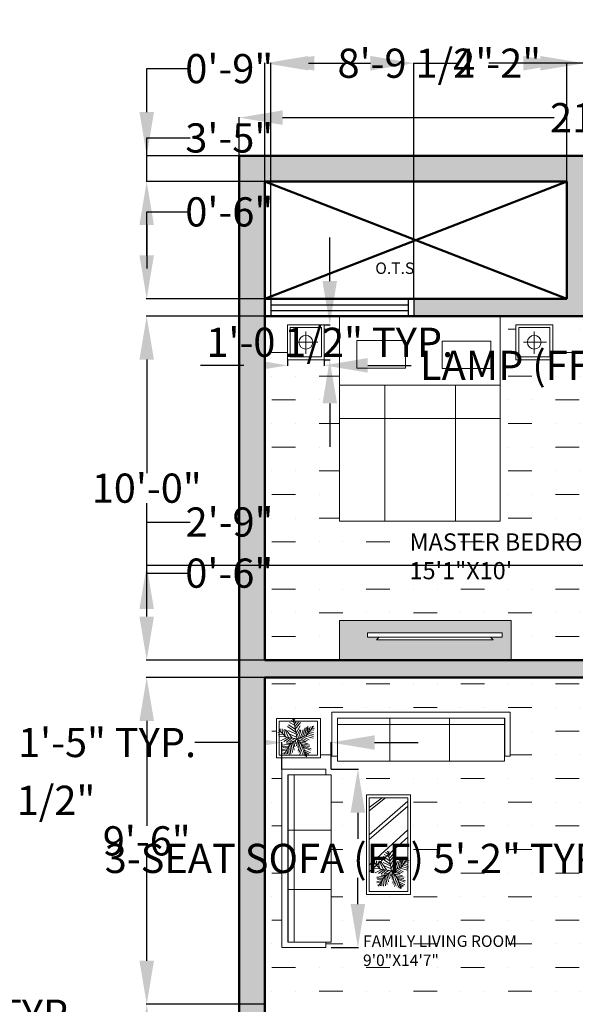
# Model space of a CAD drawing. Units: inches. Extents: x 26 to 14419, y 2 to 3479.
# Tile 8 of 9: x 14003 to 14197, y 3106 to 3449. Entities that reach past the tile are written whole.
import ezdxf

# ---------------------------------------------------------------- set-up
doc = ezdxf.new("R2010")
doc.units = ezdxf.units.IN
doc.header["$MEASUREMENT"] = 0
for name, color, linetype, lineweight in [('A-ANNO-DIMS', 2, 'Continuous', 18), ('A-AREA-IDEN', 7, 'Continuous', 18), ('A-FLOR-PATT', 252, 'Continuous', 13), ('A-FURN', 8, 'Continuous', 18), ('A-GLAZ', 3, 'Continuous', 25), ('A-WALL', 7, 'Continuous', 50), ('L-PLNT', 3, 'Continuous', 13)]:
    doc.layers.add(name, color=color, linetype=linetype, lineweight=lineweight)
doc.styles.get("Standard").update_dxf_attribs({"font": 'arial.ttf'})
doc.dimstyles.get("Standard").update_dxf_attribs({"dimtxt": 10.18, "dimasz": 15.18, "dimexe": 0.18, "dimexo": 0.0625, "dimgap": 0.09, "dimtad": 0, "dimtih": 1, "dimtoh": 1, "dimdec": 0, "dimzin": 0, "dimdsep": 46, "dimlunit": 3, "dimtxsty": 'Standard', "dimcen": 0.09, "dimadec": 0, "dimazin": 0, "dimtfac": 1, "dimtdec": 0, "dimtofl": 0, "dimtmove": 0, "dimatfit": 3, "dimfxl": 1, "dimtolj": 1, "dimtzin": 0, "dimarcsym": 0})

# ---------------------------------------------------------------- blocks, each defined once
blk = doc.blocks.new('*U5')
for p, q in [((-48.585, 21.131), (-49.309, 29.026)), ((-43.513, 28.561), (-42.427, 15.558)), ((-3.665, 19.273), (-27.574, 35.527)), ((-5.114, 28.097), (-24.676, 40.636)), ((-7.288, 39.707), (-21.778, 46.673)), ((-8.737, 47.138), (-17.069, 52.711)), ((-10.186, 53.64), (-13.084, 55.962)), ((0, 0), (-10.5, 57)), ((-9.099, 51.782), (-6.563, 55.962)), ((-7.65, 43.423), (-2.578, 49.46)), ((-5.839, 35.992), (4.667, 48.067)), ((-5.114, 27.632), (10.463, 46.673)), ((-2.941, 16.486), (8.652, 37.85)), ((16.259, 5.805), (23.142, 31.348)), ((22.055, 7.198), (27.489, 32.277)), ((27, 9), (48, 36)), ((27.127, 9.056), (31.112, 35.992)), ((31.836, 30.883), (32.561, 16.486)), ((35.096, 32.741), (37.27, 22.524)), ((38.719, 34.134), (41.979, 28.561)), ((43.791, 29.954), (51.036, 30.883)), ((44.153, 36.456), (45.239, 32.741)), ((-47.498, 19.737), (-55.83, 18.344)), ((-40.615, 13.7), (-55.105, 10.913)), ((-31.5, 4.5), (-52.5, 25.5)), ((-33.37, 6.269), (-52.207, 5.34)), ((-28.299, 3.483), (-47.86, -5.805)), ((-38.442, 26.239), (-34.819, 7.663)), ((-21.416, 3.018), (-38.079, -8.128)), ((-35.544, 28.097), (-24.314, 3.947)), ((0, 0), (-31.5, 4.5)), ((-14.533, 2.09), (-30.834, 25.31)), ((-15.982, 2.09), (-30.11, -9.521)), ((-24.314, 23.917), (-2.941, 13.7)), ((0, 0), (-22.5, -19.5)), ((-6.563, 1.161), (-21.416, -8.128)), ((-20.691, 13.7), (-1.129, 4.876)), ((-1.129, 6.734), (9.014, 26.704)), ((0, 0), (27, 9)), ((0, 0), (18, -22.5)), ((3.942, 1.625), (11.187, 24.381)), ((6.478, 1.625), (26.04, -8.592)), ((10.101, 3.483), (17.708, 26.239)), ((11.187, 3.483), (30.749, -5.805)), ((18.07, 5.805), (35.096, -3.483)), ((24.229, 7.663), (46.688, 1.625)), ((29.662, 12.307), (48.137, 6.269)), ((33.285, 16.486), (48.862, 10.913)), ((36.183, 19.737), (48.137, 17.88)), ((40.53, 25.775), (48.862, 24.846)), ((-17.431, -15.094), (-42.789, -18.809)), ((-24.314, -21.596), (-42.427, -22.06)), ((-26.849, -26.24), (-40.253, -25.775)), ((-22.5, -19.5), (-37.5, -45)), ((-15.257, -12.772), (-30.11, -12.772)), ((-25.038, -23.918), (-22.865, -45.281)), ((-20.691, -18.345), (-17.793, -44.352)), ((-6.563, -5.805), (-19.967, -9.985)), ((-17.069, -15.094), (-12.721, -40.172)), ((-13.446, -11.378), (-8.737, -32.741)), ((-9.461, -8.592), (-6.201, -23.453)), ((-4.752, -3.483), (-3.665, -14.629)), ((2.493, -3.019), (-1.491, -20.202)), ((1.769, -2.555), (24.229, -9.521)), ((5.029, -6.27), (2.131, -25.775)), ((9.014, -11.378), (3.58, -35.992)), ((14.085, -16.951), (6.478, -40.172)), ((7.565, -9.056), (32.198, -14.629)), ((18.07, -22.524), (8.289, -45.745)), ((12.274, -15.094), (36.907, -18.809)), ((16.259, -19.738), (36.183, -22.989)), ((18, -22.5), (27, -52.5)), ((18.433, -22.524), (40.53, -29.026)), ((19.157, -25.311), (38.719, -33.206)), ((-28.299, -29.026), (-42.789, -31.348)), ((-30.834, -34.135), (-42.427, -35.528)), ((-34.457, -39.708), (-40.978, -42.494)), ((-32.646, -36.921), (-31.921, -44.352)), ((-29.023, -30.884), (-27.936, -43.887)), ((20.244, -30.419), (15.897, -44.816)), ((22.78, -37.85), (19.519, -48.532)), ((21.331, -32.741), (39.081, -40.636)), ((22.78, -38.314), (34.372, -44.816)), ((24.591, -45.745), (23.142, -50.854)), ((24.591, -43.423), (30.749, -47.603)), ((26.764, -49.925), (28.213, -50.854))]:
    blk.add_line(p, q)
blk = doc.blocks.new('*D8')
at = {"layer": 'A-ANNO-DIMS', "color": 0, "lineweight": -2, "transparency": 16777216}
for p, q in [((14079.64, 3401.78), (14079.64, 3415.17)), ((14094.82, 3414.99), (14189.53, 3414.99)), ((14327.46, 3414.99), (14232.76, 3414.99)), ((14342.64, 3401.78), (14342.64, 3415.17))]:
    blk.add_line(p, q, dxfattribs=at)
at = {"layer": 'A-ANNO-DIMS', "color": 0, "transparency": 16777216}
for points in [[(14094.82, 3417.52), (14094.82, 3412.46), (14079.64, 3414.99)], [(14327.46, 3417.52), (14327.46, 3412.46), (14342.64, 3414.99)]]:
    blk.add_solid(points, dxfattribs=at)
at = {"layer": 'Defpoints', "color": 0, "transparency": 16777216}
for p in [(14342.64, 3414.99), (14079.64, 3401.72), (14342.64, 3401.72)]:
    blk.add_point(p, dxfattribs=at)
at = {"layer": 'A-ANNO-DIMS', "color": 0, "transparency": 16777216, "insert": (14211.14, 3414.99), "char_height": 10.18, "attachment_point": 5}
blk.add_mtext('\\A1;21\'-11"', dxfattribs=at)
blk = doc.blocks.new('SOFA-3SEAT-FF')
for points in [[(1.92, 15.07), (1.92, 1.81), (0, 1.81), (0, 17.18), (1.92, 17.18)], [(1.92, 17.18), (62.18, 17.18)], [(60.26, 17.18), (62.18, 17.18), (62.18, 1.81), (60.26, 1.81), (60.26, 15.07)], [(60.26, 15.07), (1.92, 15.07)]]:
    blk.add_lwpolyline(points)
blk.add_lwpolyline([(1.92, 15.02), (60.19, 15.02), (60.19, 0), (1.92, 0)], close=True)
blk = doc.blocks.new('LAMP-FF')
for p, q in [((6.41, 9.87), (6.41, 2.06)), ((2.67, 6.13), (10.62, 6.13))]:
    blk.add_line(p, q)
for points in [[(0, 12.26), (12.83, 12.26), (12.83, 0), (0, 0)], [(1, 11.26), (11.83, 11.26), (11.83, 1), (1, 1)]]:
    blk.add_lwpolyline(points, close=True)
blk.add_circle((6.41, 6.13), 2.41)
blk = doc.blocks.new('*D33')
at = {"layer": 'A-ANNO-DIMS', "color": 0, "lineweight": -2, "transparency": 16777216}
for p, q in [((14111.8, 3187.7), (14121.24, 3187.7)), ((14121.06, 3172.52), (14121.06, 3163.38)), ((14121.06, 3140.7), (14121.06, 3149.84)), ((14111.8, 3125.52), (14121.24, 3125.52))]:
    blk.add_line(p, q, dxfattribs=at)
at = {"layer": 'A-ANNO-DIMS', "color": 0, "transparency": 16777216}
for points in [[(14118.53, 3172.52), (14123.59, 3172.52), (14121.06, 3187.7)], [(14118.53, 3140.7), (14123.59, 3140.7), (14121.06, 3125.52)]]:
    blk.add_solid(points, dxfattribs=at)
at = {"layer": 'Defpoints', "color": 0, "transparency": 16777216}
for p in [(14111.74, 3187.7), (14121.06, 3187.7), (14111.74, 3125.52)]:
    blk.add_point(p, dxfattribs=at)
at = {"layer": 'A-ANNO-DIMS', "color": 0, "transparency": 16777216, "insert": (14121.06, 3156.61), "char_height": 10.18, "attachment_point": 5}
blk.add_mtext('\\A1;3-SEAT SOFA (FF) 5\'-2" TYP.', dxfattribs=at)
blk = doc.blocks.new('*D34')
at = {"layer": 'A-ANNO-DIMS', "color": 0, "lineweight": -2, "transparency": 16777216}
for p, q in [((14079.38, 3197.03), (14064.2, 3197.03)), ((14094.56, 3187.76), (14094.56, 3197.21)), ((14111.74, 3187.76), (14111.74, 3197.21)), ((14126.92, 3197.03), (14142.1, 3197.03))]:
    blk.add_line(p, q, dxfattribs=at)
at = {"layer": 'A-ANNO-DIMS', "color": 0, "transparency": 16777216}
for points in [[(14079.38, 3199.56), (14079.38, 3194.5), (14094.56, 3197.03)], [(14126.92, 3199.56), (14126.92, 3194.5), (14111.74, 3197.03)]]:
    blk.add_solid(points, dxfattribs=at)
at = {"layer": 'Defpoints', "color": 0, "transparency": 16777216}
for p in [(14094.56, 3197.03), (14094.56, 3187.7), (14111.74, 3187.7)]:
    blk.add_point(p, dxfattribs=at)
at = {"layer": 'A-ANNO-DIMS', "color": 0, "transparency": 16777216, "insert": (14033.56, 3197.03), "char_height": 10.18, "attachment_point": 5}
blk.add_mtext('\\A1;1\'-5" TYP.', dxfattribs=at)
blk = doc.blocks.new('*D37')
at = {"layer": 'A-ANNO-DIMS', "color": 0, "lineweight": -2, "transparency": 16777216}
for p, q in [((14081.32, 3328.58), (14066.14, 3328.58)), ((14096.5, 3330.45), (14096.5, 3328.4)), ((14109.33, 3330.45), (14109.33, 3328.4)), ((14124.51, 3328.58), (14139.69, 3328.58))]:
    blk.add_line(p, q, dxfattribs=at)
at = {"layer": 'A-ANNO-DIMS', "color": 0, "transparency": 16777216}
for points in [[(14081.32, 3331.11), (14081.32, 3326.05), (14096.5, 3328.58)], [(14124.51, 3331.11), (14124.51, 3326.05), (14109.33, 3328.58)]]:
    blk.add_solid(points, dxfattribs=at)
at = {"layer": 'Defpoints', "color": 0, "transparency": 16777216}
for p in [(14096.5, 3330.51), (14109.33, 3330.51), (14109.33, 3328.58)]:
    blk.add_point(p, dxfattribs=at)
at = {"layer": 'A-ANNO-DIMS', "color": 0, "transparency": 16777216, "insert": (14207.31, 3328.58), "char_height": 10.18, "attachment_point": 5}
blk.add_mtext('\\A1;LAMP (FF) 1\'-1" TYP.', dxfattribs=at)
blk = doc.blocks.new('*D38')
at = {"layer": 'A-ANNO-DIMS', "color": 0, "lineweight": -2, "transparency": 16777216}
for p, q in [((14111.25, 3357.95), (14111.25, 3373.13)), ((14109.39, 3342.77), (14111.43, 3342.77)), ((14109.39, 3330.51), (14111.43, 3330.51)), ((14111.25, 3315.33), (14111.25, 3300.15))]:
    blk.add_line(p, q, dxfattribs=at)
at = {"layer": 'A-ANNO-DIMS', "color": 0, "transparency": 16777216}
for points in [[(14108.72, 3357.95), (14113.78, 3357.95), (14111.25, 3342.77)], [(14108.72, 3315.33), (14113.78, 3315.33), (14111.25, 3330.51)]]:
    blk.add_solid(points, dxfattribs=at)
at = {"layer": 'Defpoints', "color": 0, "transparency": 16777216}
for p in [(14109.33, 3342.77), (14111.25, 3342.77), (14109.33, 3330.51)]:
    blk.add_point(p, dxfattribs=at)
at = {"layer": 'A-ANNO-DIMS', "color": 0, "transparency": 16777216, "insert": (14111.25, 3336.64), "char_height": 10.18, "attachment_point": 5}
blk.add_mtext('\\A1;1\'-0 1/2" TYP.', dxfattribs=at)
blk = doc.blocks.new('*D46')
at = {"layer": 'A-ANNO-DIMS', "color": 0, "lineweight": -2, "transparency": 16777216}
for p, q in [((13878.23, 3102.3), (13863.05, 3102.3)), ((13893.41, 3104.57), (13893.41, 3102.12)), ((13907.93, 3104.57), (13907.93, 3102.12)), ((13923.11, 3102.3), (13938.29, 3102.3))]:
    blk.add_line(p, q, dxfattribs=at)
at = {"layer": 'A-ANNO-DIMS', "color": 0, "transparency": 16777216}
for points in [[(13878.23, 3104.83), (13878.23, 3099.77), (13893.41, 3102.3)], [(13923.11, 3104.83), (13923.11, 3099.77), (13907.93, 3102.3)]]:
    blk.add_solid(points, dxfattribs=at)
at = {"layer": 'Defpoints', "color": 0, "transparency": 16777216}
for p in [(13893.41, 3104.63), (13907.93, 3104.63), (13907.93, 3102.3)]:
    blk.add_point(p, dxfattribs=at)
at = {"layer": 'A-ANNO-DIMS', "color": 0, "transparency": 16777216, "insert": (13980.79, 3102.3), "char_height": 10.18, "attachment_point": 5}
blk.add_mtext('\\A1;1\'-2 1/2" TYP.', dxfattribs=at)
blk = doc.blocks.new('*D83')
at = {"layer": 'A-ANNO-DIMS', "color": 0, "lineweight": -2, "transparency": 16777216}
for p, q in [((13953.59, 3161.69), (13953.59, 3176.87)), ((13953.59, 3176.87), (13968.77, 3176.87)), ((13883.2, 3161.69), (13953.77, 3161.69)), ((13953.59, 3142.18), (13953.59, 3146.51)), ((13883.2, 3127), (13953.77, 3127))]:
    blk.add_line(p, q, dxfattribs=at)
at = {"layer": 'A-ANNO-DIMS', "color": 0, "transparency": 16777216}
for points in [[(13951.06, 3146.51), (13956.12, 3146.51), (13953.59, 3161.69)], [(13951.06, 3142.18), (13956.12, 3142.18), (13953.59, 3127)]]:
    blk.add_solid(points, dxfattribs=at)
at = {"layer": 'Defpoints', "color": 0, "transparency": 16777216}
for p in [(13883.14, 3161.69), (13953.59, 3161.69), (13883.14, 3127)]:
    blk.add_point(p, dxfattribs=at)
at = {"layer": 'A-ANNO-DIMS', "color": 0, "transparency": 16777216, "insert": (13998.29, 3176.87), "char_height": 10.18, "attachment_point": 5}
blk.add_mtext('\\A1;2\'-10 1/2"', dxfattribs=at)
blk = doc.blocks.new('*D92')
at = {"layer": 'A-ANNO-DIMS', "color": 0, "lineweight": -2, "transparency": 16777216}
for p, q in [((14088.58, 3105.72), (14047.21, 3105.72)), ((14047.39, 3090.54), (14047.39, 3081.01)), ((14047.39, 3060.9), (14047.39, 3070.43)), ((14088.58, 3045.72), (14047.21, 3045.72))]:
    blk.add_line(p, q, dxfattribs=at)
at = {"layer": 'A-ANNO-DIMS', "color": 0, "transparency": 16777216}
for points in [[(14044.86, 3090.54), (14049.92, 3090.54), (14047.39, 3105.72)], [(14044.86, 3060.9), (14049.92, 3060.9), (14047.39, 3045.72)]]:
    blk.add_solid(points, dxfattribs=at)
at = {"layer": 'Defpoints', "color": 0, "transparency": 16777216}
for p in [(14047.39, 3105.72), (14088.64, 3105.72), (14088.64, 3045.72)]:
    blk.add_point(p, dxfattribs=at)
at = {"layer": 'A-ANNO-DIMS', "color": 0, "transparency": 16777216, "insert": (14047.39, 3075.72), "char_height": 10.18, "attachment_point": 5}
blk.add_mtext('\\A1;5\'-0"', dxfattribs=at)
blk = doc.blocks.new('*D93')
at = {"layer": 'A-ANNO-DIMS', "color": 0, "lineweight": -2, "transparency": 16777216}
for p, q in [((14088.58, 3219.75), (14047.21, 3219.75)), ((14047.39, 3204.57), (14047.39, 3168.02)), ((14047.39, 3120.9), (14047.39, 3157.44)), ((14088.58, 3105.72), (14047.21, 3105.72))]:
    blk.add_line(p, q, dxfattribs=at)
at = {"layer": 'A-ANNO-DIMS', "color": 0, "transparency": 16777216}
for points in [[(14044.86, 3204.57), (14049.92, 3204.57), (14047.39, 3219.75)], [(14044.86, 3120.9), (14049.92, 3120.9), (14047.39, 3105.72)]]:
    blk.add_solid(points, dxfattribs=at)
at = {"layer": 'Defpoints', "color": 0, "transparency": 16777216}
for p in [(14047.39, 3219.75), (14088.64, 3219.75), (14088.64, 3105.72)]:
    blk.add_point(p, dxfattribs=at)
at = {"layer": 'A-ANNO-DIMS', "color": 0, "transparency": 16777216, "insert": (14047.39, 3162.73), "char_height": 10.18, "attachment_point": 5}
blk.add_mtext('\\A1;9\'-6"', dxfattribs=at)
blk = doc.blocks.new('*D94')
at = {"layer": 'A-ANNO-DIMS', "color": 0, "lineweight": -2, "transparency": 16777216}
for p, q in [((14047.39, 3240.93), (14047.39, 3256.11)), ((14047.39, 3256.11), (14062.57, 3256.11)), ((14088.58, 3225.75), (14047.21, 3225.75)), ((14088.58, 3219.75), (14047.21, 3219.75)), ((14047.39, 3204.57), (14047.39, 3189.39))]:
    blk.add_line(p, q, dxfattribs=at)
at = {"layer": 'A-ANNO-DIMS', "color": 0, "transparency": 16777216}
for points in [[(14044.86, 3240.93), (14049.92, 3240.93), (14047.39, 3225.75)], [(14044.86, 3204.57), (14049.92, 3204.57), (14047.39, 3219.75)]]:
    blk.add_solid(points, dxfattribs=at)
at = {"layer": 'Defpoints', "color": 0, "transparency": 16777216}
for p in [(14047.39, 3225.75), (14088.64, 3225.75), (14088.64, 3219.75)]:
    blk.add_point(p, dxfattribs=at)
at = {"layer": 'A-ANNO-DIMS', "color": 0, "transparency": 16777216, "insert": (14076.19, 3256.11), "char_height": 10.18, "attachment_point": 5}
blk.add_mtext('\\A1;0\'-6"', dxfattribs=at)
blk = doc.blocks.new('*D95')
at = {"layer": 'A-ANNO-DIMS', "color": 0, "lineweight": -2, "transparency": 16777216}
for p, q in [((14088.58, 3345.75), (14047.21, 3345.75)), ((14047.39, 3330.57), (14047.39, 3291.03)), ((14047.39, 3240.93), (14047.39, 3280.46)), ((14088.58, 3225.75), (14047.21, 3225.75))]:
    blk.add_line(p, q, dxfattribs=at)
at = {"layer": 'A-ANNO-DIMS', "color": 0, "transparency": 16777216}
for points in [[(14044.86, 3330.57), (14049.92, 3330.57), (14047.39, 3345.75)], [(14044.86, 3240.93), (14049.92, 3240.93), (14047.39, 3225.75)]]:
    blk.add_solid(points, dxfattribs=at)
at = {"layer": 'Defpoints', "color": 0, "transparency": 16777216}
for p in [(14047.39, 3345.75), (14088.64, 3345.75), (14088.64, 3225.75)]:
    blk.add_point(p, dxfattribs=at)
at = {"layer": 'A-ANNO-DIMS', "color": 0, "transparency": 16777216, "insert": (14047.39, 3285.75), "char_height": 10.18, "attachment_point": 5}
blk.add_mtext('\\A1;10\'-0"', dxfattribs=at)
blk = doc.blocks.new('*D96')
at = {"layer": 'A-ANNO-DIMS', "color": 0, "lineweight": -2, "transparency": 16777216}
for p, q in [((14047.39, 3366.93), (14047.39, 3382.11)), ((14047.39, 3382.11), (14062.57, 3382.11)), ((14088.58, 3351.75), (14047.21, 3351.75)), ((14088.58, 3345.75), (14047.21, 3345.75)), ((14047.39, 3330.57), (14047.39, 3315.39))]:
    blk.add_line(p, q, dxfattribs=at)
at = {"layer": 'A-ANNO-DIMS', "color": 0, "transparency": 16777216}
for points in [[(14044.86, 3366.93), (14049.92, 3366.93), (14047.39, 3351.75)], [(14044.86, 3330.57), (14049.92, 3330.57), (14047.39, 3345.75)]]:
    blk.add_solid(points, dxfattribs=at)
at = {"layer": 'Defpoints', "color": 0, "transparency": 16777216}
for p in [(14047.39, 3351.75), (14088.64, 3351.75), (14088.64, 3345.75)]:
    blk.add_point(p, dxfattribs=at)
at = {"layer": 'A-ANNO-DIMS', "color": 0, "transparency": 16777216, "insert": (14076.19, 3382.11), "char_height": 10.18, "attachment_point": 5}
blk.add_mtext('\\A1;0\'-6"', dxfattribs=at)
blk = doc.blocks.new('*D97')
at = {"layer": 'A-ANNO-DIMS', "color": 0, "lineweight": -2, "transparency": 16777216}
for p, q in [((14047.39, 3392.72), (14047.39, 3407.9)), ((14047.39, 3407.9), (14062.57, 3407.9)), ((14088.58, 3392.72), (14047.21, 3392.72)), ((14047.39, 3366.93), (14047.39, 3377.54)), ((14088.58, 3351.75), (14047.21, 3351.75))]:
    blk.add_line(p, q, dxfattribs=at)
at = {"layer": 'A-ANNO-DIMS', "color": 0, "transparency": 16777216}
for points in [[(14044.86, 3377.54), (14049.92, 3377.54), (14047.39, 3392.72)], [(14044.86, 3366.93), (14049.92, 3366.93), (14047.39, 3351.75)]]:
    blk.add_solid(points, dxfattribs=at)
at = {"layer": 'Defpoints', "color": 0, "transparency": 16777216}
for p in [(14047.39, 3392.72), (14088.64, 3392.72), (14088.64, 3351.75)]:
    blk.add_point(p, dxfattribs=at)
at = {"layer": 'A-ANNO-DIMS', "color": 0, "transparency": 16777216, "insert": (14076.19, 3407.9), "char_height": 10.18, "attachment_point": 5}
blk.add_mtext('\\A1;3\'-5"', dxfattribs=at)
blk = doc.blocks.new('*D98')
at = {"layer": 'A-ANNO-DIMS', "color": 0, "lineweight": -2, "transparency": 16777216}
for p, q in [((14047.39, 3416.9), (14047.39, 3432.08)), ((14047.39, 3432.08), (14062.57, 3432.08)), ((14079.58, 3401.72), (14047.21, 3401.72)), ((14088.58, 3392.72), (14047.21, 3392.72)), ((14047.39, 3377.54), (14047.39, 3362.36))]:
    blk.add_line(p, q, dxfattribs=at)
at = {"layer": 'A-ANNO-DIMS', "color": 0, "transparency": 16777216}
for points in [[(14044.86, 3416.9), (14049.92, 3416.9), (14047.39, 3401.72)], [(14044.86, 3377.54), (14049.92, 3377.54), (14047.39, 3392.72)]]:
    blk.add_solid(points, dxfattribs=at)
at = {"layer": 'Defpoints', "color": 0, "transparency": 16777216}
for p in [(14047.39, 3401.72), (14079.64, 3401.72), (14088.64, 3392.72)]:
    blk.add_point(p, dxfattribs=at)
at = {"layer": 'A-ANNO-DIMS', "color": 0, "transparency": 16777216, "insert": (14076.19, 3432.08), "char_height": 10.18, "attachment_point": 5}
blk.add_mtext('\\A1;0\'-9"', dxfattribs=at)
blk = doc.blocks.new('*D106')
at = {"layer": 'A-ANNO-DIMS', "color": 0, "lineweight": -2, "transparency": 16777216}
for p, q in [((14088.64, 3392.78), (14088.64, 3434.15)), ((14103.82, 3433.97), (14115.8, 3433.97)), ((14178.75, 3433.97), (14166.77, 3433.97)), ((14193.93, 3392.78), (14193.93, 3434.15))]:
    blk.add_line(p, q, dxfattribs=at)
at = {"layer": 'A-ANNO-DIMS', "color": 0, "transparency": 16777216}
for points in [[(14103.82, 3436.5), (14103.82, 3431.44), (14088.64, 3433.97)], [(14178.75, 3436.5), (14178.75, 3431.44), (14193.93, 3433.97)]]:
    blk.add_solid(points, dxfattribs=at)
at = {"layer": 'Defpoints', "color": 0, "transparency": 16777216}
for p in [(14193.93, 3433.97), (14088.64, 3392.72), (14193.93, 3392.72)]:
    blk.add_point(p, dxfattribs=at)
at = {"layer": 'A-ANNO-DIMS', "color": 0, "transparency": 16777216, "insert": (14141.28, 3433.97), "char_height": 10.18, "attachment_point": 5}
blk.add_mtext('\\A1;8\'-9 1/2"', dxfattribs=at)
blk = doc.blocks.new('*D107')
at = {"layer": 'A-ANNO-DIMS', "color": 0, "lineweight": -2, "transparency": 16777216}
for p, q in [((14184.75, 3433.97), (14169.57, 3433.97)), ((14199.93, 3392.78), (14199.93, 3434.15)), ((14257.64, 3392.78), (14257.64, 3434.15)), ((14272.82, 3433.97), (14288, 3433.97))]:
    blk.add_line(p, q, dxfattribs=at)
at = {"layer": 'A-ANNO-DIMS', "color": 0, "transparency": 16777216}
for points in [[(14184.75, 3436.5), (14184.75, 3431.44), (14199.93, 3433.97)], [(14272.82, 3436.5), (14272.82, 3431.44), (14257.64, 3433.97)]]:
    blk.add_solid(points, dxfattribs=at)
at = {"layer": 'Defpoints', "color": 0, "transparency": 16777216}
for p in [(14257.64, 3433.97), (14199.93, 3392.72), (14257.64, 3392.72)]:
    blk.add_point(p, dxfattribs=at)
at = {"layer": 'A-ANNO-DIMS', "color": 0, "transparency": 16777216, "insert": (14228.78, 3433.97), "char_height": 10.18, "attachment_point": 5}
blk.add_mtext('\\A1;4\'-9 1/2"', dxfattribs=at)
blk = doc.blocks.new('*D109')
at = {"layer": 'A-ANNO-DIMS', "color": 0, "lineweight": -2, "transparency": 16777216}
for p, q in [((14199.604862, 3433.969118), (14184.424862, 3433.969118)), ((14214.784862, 3401.781618), (14214.784862, 3434.149118)), ((14242.784862, 3401.781618), (14242.784862, 3434.149118)), ((14257.964862, 3433.969118), (14273.144862, 3433.969118))]:
    blk.add_line(p, q, dxfattribs=at)
at = {"layer": 'A-ANNO-DIMS', "color": 0, "transparency": 16777216}
for points in [[(14199.604862, 3436.499118), (14199.604862, 3431.439118), (14214.784862, 3433.969118)], [(14257.964862, 3436.499118), (14257.964862, 3431.439118), (14242.784862, 3433.969118)]]:
    blk.add_solid(points, dxfattribs=at)
at = {"layer": 'Defpoints', "color": 0, "transparency": 16777216}
for p in [(14242.784862, 3433.969118), (14214.784862, 3401.719118), (14242.784862, 3401.719118)]:
    blk.add_point(p, dxfattribs=at)
at = {"layer": 'A-ANNO-DIMS', "color": 0, "transparency": 16777216, "insert": (14228.784862, 3433.969118), "char_height": 10.18, "attachment_point": 5}
blk.add_mtext('\\A1;2\'-4"', dxfattribs=at)
blk = doc.blocks.new('*D115')
at = {"layer": 'A-ANNO-DIMS', "color": 0, "lineweight": -2, "transparency": 16777216}
for p, q in [((14090.64, 3351.81), (14090.64, 3434.15)), ((14105.82, 3433.97), (14125.46, 3433.97)), ((14140.64, 3351.81), (14140.64, 3434.15)), ((14140.64, 3433.97), (14155.82, 3433.97))]:
    blk.add_line(p, q, dxfattribs=at)
at = {"layer": 'A-ANNO-DIMS', "color": 0, "transparency": 16777216}
for points in [[(14105.82, 3436.5), (14105.82, 3431.44), (14090.64, 3433.97)], [(14125.46, 3436.5), (14125.46, 3431.44), (14140.64, 3433.97)]]:
    blk.add_solid(points, dxfattribs=at)
at = {"layer": 'Defpoints', "color": 0, "transparency": 16777216}
for p in [(14140.64, 3433.97), (14090.64, 3351.75), (14140.64, 3351.75)]:
    blk.add_point(p, dxfattribs=at)
at = {"layer": 'A-ANNO-DIMS', "color": 0, "transparency": 16777216, "insert": (14169.65, 3433.97), "char_height": 10.18, "attachment_point": 5}
blk.add_mtext('\\A1;4\'-2"', dxfattribs=at)
blk = doc.blocks.new('*D118')
at = {"layer": 'A-ANNO-DIMS', "color": 0, "lineweight": -2, "transparency": 16777216}
for p, q in [((14202.46, 3433.97), (14187.28, 3433.97)), ((14217.64, 3164.78), (14217.64, 3434.15)), ((14227.64, 3164.78), (14227.64, 3434.15)), ((14242.82, 3433.97), (14258, 3433.97))]:
    blk.add_line(p, q, dxfattribs=at)
at = {"layer": 'A-ANNO-DIMS', "color": 0, "transparency": 16777216}
for points in [[(14202.46, 3436.5), (14202.46, 3431.44), (14217.64, 3433.97)], [(14242.82, 3436.5), (14242.82, 3431.44), (14227.64, 3433.97)]]:
    blk.add_solid(points, dxfattribs=at)
at = {"layer": 'Defpoints', "color": 0, "transparency": 16777216}
for p in [(14227.64, 3433.97), (14217.64, 3164.72), (14227.64, 3164.72)]:
    blk.add_point(p, dxfattribs=at)
at = {"layer": 'A-ANNO-DIMS', "color": 0, "transparency": 16777216, "insert": (14275.58, 3433.97), "char_height": 10.18, "attachment_point": 5}
blk.add_mtext('\\A1;0\'-10"', dxfattribs=at)
blk = doc.blocks.new('*D120')
at = {"layer": 'A-ANNO-DIMS', "color": 0, "lineweight": -2, "transparency": 16777216}
for p, q in [((14047.39, 3258.75), (14047.39, 3273.93)), ((14047.39, 3273.93), (14062.57, 3273.93)), ((14254.58, 3258.75), (14047.21, 3258.75)), ((14047.39, 3240.93), (14047.39, 3243.57)), ((14257.58, 3225.75), (14047.21, 3225.75))]:
    blk.add_line(p, q, dxfattribs=at)
at = {"layer": 'A-ANNO-DIMS', "color": 0, "transparency": 16777216}
for points in [[(14044.86, 3243.57), (14049.92, 3243.57), (14047.39, 3258.75)], [(14044.86, 3240.93), (14049.92, 3240.93), (14047.39, 3225.75)]]:
    blk.add_solid(points, dxfattribs=at)
at = {"layer": 'Defpoints', "color": 0, "transparency": 16777216}
for p in [(14047.39, 3258.75), (14254.64, 3258.75), (14257.64, 3225.75)]:
    blk.add_point(p, dxfattribs=at)
at = {"layer": 'A-ANNO-DIMS', "color": 0, "transparency": 16777216, "insert": (14076.28, 3273.93), "char_height": 10.18, "attachment_point": 5}
blk.add_mtext('\\A1;2\'-9"', dxfattribs=at)

msp = doc.modelspace()

# ---------------------------------------------------------------- hatches: boundary and pattern name
at = {"layer": 'A-FLOR-PATT'}
h = msp.add_hatch(color=256, dxfattribs=at)
h.dxf.hatch_style = 1
h.paths.add_polyline_path([(13922.09, 3432), (13659.09, 3432), (13659.09, 2842), (13668.09, 2842), (13668.09, 2851), (13668.09, 2899), (13668.09, 2908), (13668.09, 3076), (13706.09, 3076), (13706.09, 3085), (13668.09, 3085), (13668.09, 3249), (13712.76, 3249), (13712.76, 3255), (13668.09, 3255), (13668.09, 3375), (13720.94, 3375), (13720.94, 3378, -0.017236), (13720.94, 3380), (13720.94, 3381), (13668.09, 3381), (13668.09, 3423), (13784.09, 3423), (13784.09, 3381), (13753.94, 3381), (13753.94, 3375), (13784.09, 3375), (13784.09, 3255), (13758.77, 3255), (13758.77, 3249), (13784.09, 3249), (13793.09, 3249), (13793.09, 3255), (13793.09, 3423), (13913.09, 3423), (13913.09, 3255), (13832.09, 3255), (13832.09, 3254, -0.014283), (13832.09, 3252), (13832.09, 3249), (13836.57, 3249), (13836.57, 3234), (13839.57, 3234, -0.017236), (13841.57, 3234), (13842.57, 3234), (13842.57, 3249), (13913.09, 3249), (13913.09, 3201), (13892.46, 3201), (13793.09, 3201), (13784.09, 3201), (13784.09, 3195), (13793.09, 3195), (13913.09, 3195), (13913.09, 3127), (13922.09, 3127)])
h.paths.add_polyline_path([(13922.09, 3013.5), (13913.09, 3013.5), (13913.09, 2908), (13892.09, 2908), (13892.09, 2899), (13913.09, 2899), (13913.09, 2851), (13793.09, 2851), (13784.09, 2851), (13784.09, 2842), (13922.09, 2842)], flags=17)
h.paths.add_polyline_path([(13793.09, 3085), (13784.09, 3085), (13784.09, 3076), (13784.09, 3071.08), (13784.09, 3066.17), (13784.09, 2908), (13784.09, 2899.07), (13793.09, 2899), (13802.09, 2899), (13814.09, 2899), (13814.09, 2908), (13793.09, 2908)], flags=17)
h.paths.add_polyline_path([(14342.64, 3401.72), (14242.78, 3401.72), (14242.78, 3392.72), (14257.64, 3392.72), (14257.64, 3351.75), (14257.64, 3345.75), (14257.64, 3330.73), (14263.64, 3330.73), (14263.64, 3392.72), (14333.64, 3392.72), (14333.64, 3284.72), (14302.92, 3284.72), (14302.92, 3281.72, -0.022645), (14302.92, 3279.12), (14302.92, 3278.72), (14333.64, 3278.72), (14333.64, 3170.72), (14316.1, 3170.72), (14263.64, 3170.72), (14263.64, 3278.72), (14269.92, 3278.72), (14269.92, 3284.72), (14263.64, 3284.72), (14257.64, 3284.72), (14257.64, 3225.75), (14257.64, 3219.75), (14257.64, 3164.72), (14333.64, 3164.72), (14333.64, 3110.37), (14210.01, 3110.37), (14210.01, 3104.37), (14257.64, 3104.37), (14257.64, 3024), (14263.64, 3024), (14263.64, 3039.72), (14263.64, 3104.37), (14333.64, 3104.37), (14333.64, 3045.72), (14333.64, 3039.72), (14333.64, 2967.72), (14296.64, 2967.72), (14296.64, 2964.72, -0.017236), (14296.64, 2962.72), (14296.64, 2961.72), (14333.64, 2961.72), (14333.64, 2882.72), (14312.64, 2882.72), (14312.64, 2873.72), (14333.64, 2873.72), (14333.64, 2820.72), (14333.64, 2811.72), (14342.64, 2811.72)])
h.paths.add_polyline_path([(14088.64, 3219.75), (14218.64, 3219.75), (14218.64, 3222.75, -0.014283), (14218.64, 3224.75), (14218.64, 3225.75), (14088.64, 3225.75), (14088.64, 3345.75), (14088.64, 3351.75), (14088.64, 3392.72), (14193.93, 3392.72), (14193.93, 3351.75), (14140.64, 3351.75), (14140.64, 3345.75), (14170.7, 3345.75), (14218.64, 3345.75), (14218.64, 3348.75, -0.014283), (14218.64, 3350.75), (14218.64, 3351.75), (14199.93, 3351.75), (14199.93, 3392.72), (14214.78, 3392.72), (14214.78, 3401.72), (14079.64, 3401.72), (14079.64, 2811.72), (14088.64, 2811.72), (14088.64, 2820.72), (14088.64, 2873.72), (14116.21, 2873.72), (14116.21, 2876.57), (14116.21, 2882.72), (14088.64, 2882.72), (14088.64, 3039.72), (14216.01, 3039.72), (14216.01, 3065.37), (14215.01, 3065.37, -0.014283), (14213.01, 3065.37), (14210.01, 3065.37), (14210.01, 3045.72), (14154.64, 3045.72), (14148.64, 3045.72), (14088.64, 3045.72)])
h.paths.add_polyline_path([(14284.64, 2882.72), (14263.64, 2882.72), (14263.64, 2961.72), (14263.64, 2967.72), (14257.64, 2967.72), (14257.64, 2956.69), (14257.64, 2916.18), (14257.64, 2882.72), (14249.61, 2882.72), (14249.61, 2873.72), (14284.64, 2873.72)], flags=17)
h.paths.add_polyline_path([(14202.78, 2882.72), (14189.55, 2882.72), (14189.55, 2879.95), (14189.55, 2873.72), (14202.78, 2873.72)], flags=17)
h = msp.add_hatch(dxfattribs=at)
h.set_pattern_fill('MUDST', color=256, scale=33)
h.paths.add_polyline_path([(14304.4, 3368.55), (14263.64, 3368.55), (14263.64, 3330.73), (14257.64, 3330.73), (14257.64, 3345.75), (14254.64, 3345.75), (14254.64, 3348.75), (14252.64, 3348.75), (14252.64, 3384.75, 0.397579), (14218.64, 3350.75), (14218.64, 3345.75), (14170.7, 3345.75), (14170.7, 3274.26), (14114.64, 3274.26), (14114.64, 3345.75), (14088.64, 3345.75), (14088.64, 3225.75), (14114.67, 3225.75), (14114.67, 3239.54), (14174.56, 3239.54), (14174.56, 3225.75), (14218.69, 3225.75, -0.405865), (14254.64, 3258.75), (14254.64, 3225.75), (14257.64, 3225.75), (14257.64, 3284.72), (14263.64, 3284.72), (14272.92, 3284.72), (14272.92, 3281.72), (14274.92, 3281.72), (14274.92, 3251.72, 0.394163), (14302.92, 3279.12), (14302.92, 3284.72), (14304.4, 3284.72)])
h.paths.add_polyline_path([(14189.03, 3330.51), (14176.2, 3330.51), (14176.2, 3342.77), (14189.03, 3342.77)], flags=16)
h.paths.add_polyline_path([(14188.03, 3331.51), (14177.21, 3331.51), (14177.21, 3341.77), (14188.03, 3341.77)], flags=0)
h.paths.add_polyline_path([(14185.02, 3336.64, -1), (14180.21, 3336.64, -1)], flags=0)
h.paths.add_polyline_path([(14109.33, 3330.51), (14096.5, 3330.51), (14096.5, 3342.77), (14109.33, 3342.77)], flags=16)
h.paths.add_polyline_path([(14108.33, 3331.51), (14097.5, 3331.51), (14097.5, 3341.77), (14108.33, 3341.77)], flags=0)
h.paths.add_polyline_path([(14105.32, 3336.64, -1), (14100.51, 3336.64, -1)], flags=0)
h.paths.add_polyline_path([(14257.64, 3219.75), (14254.64, 3219.75), (14254.64, 3222.75), (14252.64, 3222.75), (14252.64, 3258.75, 0.397579), (14218.64, 3224.75), (14218.64, 3219.75), (14088.64, 3219.75), (14088.64, 3105.72), (14154.64, 3105.72), (14154.64, 3045.72), (14210.01, 3045.72), (14210.01, 3065.37), (14215.01, 3065.37, 0.397579), (14249.01, 3099.37), (14213.01, 3099.37), (14213.01, 3101.37), (14210.01, 3101.37), (14210.01, 3110.37), (14217.64, 3110.37), (14217.64, 3164.72), (14215.11, 3164.72), (14215.11, 3170.72), (14257.64, 3170.72)])
h.paths.add_polyline_path([(14174.2, 3192.28), (14172.21, 3192.28), (14172.21, 3190.47), (14113.94, 3190.47), (14113.94, 3192.28), (14112.02, 3192.28), (14112.02, 3207.65), (14113.94, 3207.65), (14174.2, 3207.65)], flags=16)
h.paths.add_polyline_path([(14132.26, 3203.31), (14132.26, 3205.54), (14153.01, 3205.54), (14153.01, 3203.31)], flags=0)
h.paths.add_polyline_path([(14139.45, 3178.77), (14139.45, 3144.03), (14124.04, 3144.03), (14124.04, 3178.77)], flags=16)
h.paths.add_polyline_path([(14138.45, 3177.77), (14138.45, 3145.03), (14125.04, 3145.03), (14125.04, 3177.77)], flags=0)
h.paths.add_polyline_path([(14127.62, 3154.26), (14127.69, 3154.32), (14127.65, 3154.8), (14127.17, 3154.71)], flags=0)
h.paths.add_polyline_path([(14137.62, 3155.43), (14138.07, 3155.38), (14137.86, 3155.74)], flags=0)
h.paths.add_polyline_path([(14134.11, 3152.76), (14134.62, 3152.52), (14134.75, 3152.98)], flags=0)
h.paths.add_polyline_path([(14134.97, 3149.61), (14135.06, 3149.3), (14135.3, 3149.21), (14134.97, 3149.61)], flags=0)
h.paths.add_polyline_path([(14129.06, 3148.22), (14128.85, 3148.19), (14128.88, 3147.91)], flags=0)
h.paths.add_polyline_path([(14129.76, 3149.73), (14129.77, 3149.7), (14129.81, 3149.73)], flags=0)
h.paths.add_polyline_path([(14129.81, 3152.94), (14129.51, 3152.8), (14129.91, 3152.74)], flags=0)
h.paths.add_polyline_path([(14129.97, 3154.13), (14131.4, 3152.09), (14132.47, 3152.75), (14132.58, 3152.96)], flags=0)
h.paths.add_polyline_path([(14131.76, 3158.63), (14131.62, 3158.74), (14131.67, 3158.49)], flags=0)
h.paths.add_polyline_path([(14133.11, 3151.99), (14133.11, 3152.01), (14133.11, 3151.99)], flags=0)
h.paths.add_polyline_path([(14135.18, 3148.48), (14135.04, 3148), (14135.53, 3147.73), (14135.69, 3148.25)], flags=0)
h.paths.add_polyline_path([(14111.74, 3127.44), (14109.92, 3127.44), (14109.92, 3125.52), (14094.56, 3125.52), (14094.56, 3127.44), (14094.56, 3187.7), (14109.92, 3187.7), (14109.92, 3185.71), (14111.74, 3185.71)], flags=16)
h.paths.add_polyline_path([(14098.89, 3166.51), (14098.89, 3145.76), (14096.67, 3145.76), (14096.67, 3166.51)], flags=0)
h.paths.add_polyline_path([(14107.98, 3191.64), (14092.66, 3191.64), (14092.66, 3205.45), (14107.98, 3205.45)], flags=16)
h.paths.add_polyline_path([(14102.61, 3192.64), (14102.72, 3192.57), (14102.74, 3192.64)], flags=0)
h.paths.add_polyline_path([(14101.15, 3198.79), (14101.66, 3198.55), (14101.79, 3199)], flags=0)
h.paths.add_polyline_path([(14105.37, 3201.99), (14105.29, 3202.26), (14105.04, 3201.95)], flags=0)
h.paths.add_polyline_path([(14102.01, 3195.63), (14102.11, 3195.33), (14102.34, 3195.23), (14102.02, 3195.64)], flags=0)
h.paths.add_polyline_path([(14102.22, 3194.5), (14102.08, 3194.03), (14102.57, 3193.75), (14102.73, 3194.27)], flags=0)
h.paths.add_polyline_path([(14096.1, 3194.24), (14095.89, 3194.22), (14095.92, 3193.93)], flags=0)
h.paths.add_polyline_path([(14096.81, 3195.75), (14096.81, 3195.72), (14096.85, 3195.75)], flags=0)
h.paths.add_polyline_path([(14094.74, 3200.21), (14094.69, 3200.82), (14094.21, 3200.74)], flags=0)
h.paths.add_polyline_path([(14096.86, 3198.97), (14096.55, 3198.82), (14096.95, 3198.77)], flags=0)
h.paths.add_polyline_path([(14097.01, 3200.16), (14098.44, 3198.11), (14099.51, 3198.78), (14099.62, 3198.98)], flags=0)
h.paths.add_polyline_path([(14098.8, 3204.66), (14098.66, 3204.77), (14098.71, 3204.51)], flags=0)
h.paths.add_polyline_path([(14100.15, 3198.02), (14100.15, 3198.03), (14100.15, 3198.02)], flags=0)
h.paths.add_polyline_path([(14257.64, 2967.72), (14263.64, 2967.72), (14266.64, 2967.72), (14296.64, 2967.72), (14304.52, 2967.72), (14304.52, 3072.04), (14263.64, 3072.04), (14263.64, 3039.72), (14263.64, 3024), (14257.64, 3024), (14257.64, 3104.37), (14216.01, 3104.37), (14216.01, 3101.37), (14249.01, 3101.37, -0.405865), (14216.01, 3065.41), (14216.01, 3039.72), (14088.64, 3039.72), (14088.64, 3034.24), (14107.2, 3034.24), (14107.2, 3010.33), (14088.64, 3010.33), (14088.64, 3001.38), (14176.64, 3001.38), (14176.64, 2931.05), (14088.64, 2931.05), (14088.64, 2926.95), (14107.2, 2926.95), (14107.2, 2903.04), (14088.64, 2903.04), (14088.64, 2882.72), (14116.21, 2882.72), (14116.21, 2876.57), (14151.84, 2876.57), (14151.84, 2882.72), (14189.55, 2882.72), (14257.64, 2882.72), (14257.64, 2916.18), (14244.9, 2916.18), (14244.9, 2956.69), (14257.64, 2956.69)])
h.paths.add_polyline_path([(14199.2, 2873.72), (14189.55, 2873.72), (14189.55, 2879.95), (14151.84, 2879.95), (14151.84, 2873.72), (14116.21, 2873.72), (14088.64, 2873.72), (14088.64, 2820.72), (14088.64, 2813.09), (14199.2, 2813.09)])
h.paths.add_polyline_path([(14272.13, 3336.81), (14293.39, 3336.81), (14293.39, 3351.73), (14272.13, 3351.73)], flags=24)
h.paths.add_polyline_path([(14208.53, 3375.98), (14237.24, 3375.98), (14237.24, 3384.22), (14208.53, 3384.22)], flags=25)
h.paths.add_polyline_path([(14136.68, 3250.57), (14220.54, 3250.57), (14220.54, 3272.96), (14136.68, 3272.96)], flags=24)
h.paths.add_polyline_path([(14121.4, 3116.81), (14182.4, 3116.81), (14182.4, 3131.73), (14121.4, 3131.73)], flags=24)
h.paths.add_polyline_path([(14268.29, 3033.43), (14289.54, 3033.43), (14289.54, 3048.36), (14268.29, 3048.36)], flags=24)
h.paths.add_polyline_path([(14151.68, 2960.42), (14207.58, 2960.42), (14207.58, 2975.35), (14151.68, 2975.35)], flags=25)
h.paths.add_polyline_path([(14128.74, 2839.15), (14157.44, 2839.15), (14157.44, 2847.39), (14128.74, 2847.39)], flags=24)
h = msp.add_hatch(color=256, dxfattribs=at)
h.dxf.hatch_style = 1
h.paths.add_polyline_path([(14174.56, 3239.54), (14114.67, 3239.54), (14114.67, 3225.75), (14174.56, 3225.75)])
h.paths.add_polyline_path([(14171.37, 3235.3), (14171.37, 3233.8), (14167.29, 3233.8), (14168.29, 3232.84), (14127.56, 3232.84), (14128.52, 3233.8), (14124.42, 3233.8), (14124.42, 3235.3)], flags=16)

# ---------------------------------------------------------------- linework, layer by layer
at = {"layer": 'A-FURN'}
for p, q in [((14114.64, 3321.68), (14170.7, 3321.68)), ((14130.5, 3321.68), (14130.5, 3274.26)), ((14155.11, 3321.68), (14155.11, 3274.26)), ((14114.64, 3310), (14170.7, 3310)), ((14128.52, 3233.8), (14127.56, 3232.84)), ((14127.56, 3232.84), (14168.29, 3232.84)), ((14168.29, 3232.84), (14167.29, 3233.8)), ((14132.26, 3205.49), (14132.26, 3190.47)), ((14153.01, 3205.49), (14153.01, 3190.47)), ((14113.94, 3203.31), (14172.21, 3203.31)), ((14098.89, 3127.44), (14098.89, 3185.71)), ((14129.52, 3177.77), (14125.04, 3174.42)), ((14130.73, 3177.77), (14125.04, 3173.24)), ((14138.45, 3176.62), (14125.04, 3164.86)), ((14138.45, 3174.79), (14125.04, 3163.17)), ((14096.72, 3166.51), (14111.74, 3166.51)), ((14138.45, 3166.58), (14125.04, 3154.29)), ((14138.45, 3164.01), (14125.04, 3151.93)), ((14096.72, 3145.76), (14111.74, 3145.76))]:
    msp.add_line(p, q, dxfattribs=at)
for points in [[(14114.64, 3345.75), (14170.7, 3345.75), (14170.7, 3274.26), (14114.64, 3274.26)], [(14120.72, 3337.22), (14137.7, 3337.22), (14137.7, 3327.63), (14120.72, 3327.63)], [(14150.53, 3337.05), (14167.51, 3337.05), (14167.51, 3327.46), (14150.53, 3327.46)], [(14114.67, 3225.75), (14174.56, 3225.75), (14174.56, 3239.54), (14114.67, 3239.54)], [(14124.42, 3233.8), (14171.37, 3233.8), (14171.37, 3235.3), (14124.42, 3235.3)], [(14092.66, 3205.45), (14107.98, 3205.45), (14107.98, 3191.64), (14092.66, 3191.64)], [(14093.66, 3204.45), (14106.98, 3204.45), (14106.98, 3192.64), (14093.66, 3192.64)], [(14124.04, 3178.77), (14139.45, 3178.77), (14139.45, 3144.03), (14124.04, 3144.03)], [(14125.04, 3177.77), (14138.45, 3177.77), (14138.45, 3145.03), (14125.04, 3145.03)]]:
    msp.add_lwpolyline(points, close=True, dxfattribs=at)
at = {"layer": 'A-GLAZ'}
for p, q in [((14090.64, 3351.75), (14090.64, 3345.75)), ((14090.64, 3349.75), (14138.64, 3349.75)), ((14138.64, 3351.75), (14138.64, 3345.75)), ((14140.64, 3351.75), (14140.64, 3345.75)), ((14090.64, 3347.75), (14138.64, 3347.75))]:
    msp.add_line(p, q, dxfattribs=at)
at = {"layer": 'A-WALL'}
for p, q in [((14079.64, 2811.72), (14079.64, 3401.72)), ((14079.64, 3401.72), (14342.64, 3401.72)), ((14088.64, 3392.72), (14193.93, 3392.72)), ((14088.64, 3351.75), (14088.64, 3392.72)), ((14088.64, 3392.72), (14193.93, 3351.75)), ((14193.93, 3392.72), (14088.64, 3351.75)), ((14193.93, 3351.75), (14193.93, 3392.72)), ((14088.64, 3351.75), (14193.93, 3351.75)), ((14088.64, 3351.75), (14088.64, 3345.75)), ((14088.64, 3345.75), (14218.64, 3345.75)), ((14088.64, 3225.75), (14088.64, 3345.75)), ((14088.64, 3225.75), (14218.69, 3225.75)), ((14088.64, 3219.75), (14218.64, 3219.75)), ((14088.64, 3045.72), (14088.64, 3219.75))]:
    msp.add_line(p, q, dxfattribs=at)

# ---------------------------------------------------------------- block references
at = {"layer": 'A-FURN'}
for name, p in [('LAMP-FF', (14096.5, 3330.51)), ('LAMP-FF', (14176.2, 3330.51)), ('SOFA-3SEAT-FF', (14112.02, 3190.47))]:
    msp.add_blockref(name, p, dxfattribs=at)
at = {"layer": 'A-FURN', "rotation": 90.00000000000365}
msp.add_blockref('SOFA-3SEAT-FF', (14111.74, 3125.52), dxfattribs=at)
at = {"layer": 'L-PLNT', "xscale": 0.1202515193595938, "yscale": 0.1202515193595938, "zscale": 0.1202515193595938}
for p in [(14099.84, 3198.35), (14132.8, 3152.33)]:
    msp.add_blockref('*U5', p, dxfattribs=at)

# ---------------------------------------------------------------- texts
at = {"layer": 'A-AREA-IDEN', "attachment_point": 1}
for s, width, insert, char_height in [('O.T.S', 7.6086, (14127.13, 3364.47), 4), ('MASTER BEDROOM\\P15\'1"X10\'', 89.8665, (14139.09, 3269.98), 6), ('FAMILY LIVING ROOM\\P9\'0"X14\'7"', 62.3086, (14122.86, 3129.75), 4)]:
    msp.add_mtext_dynamic_manual_height_columns(s, width=width, gutter_width=1, heights=[0], dxfattribs=dict(at, insert=insert, char_height=char_height))

# ---------------------------------------------------------------- dimensions: what is measured, and where the dimension line sits
at = {"layer": 'A-ANNO-DIMS'}
for base, p1, p2, override, picture, middle in [((14193.93, 3433.97), (14088.64, 3392.72), (14193.93, 3392.72), {"dimdec": 1, "dimlfac": 1, "dimrnd": 0, "dimzin": 1, "dimdsep": 46, "dimlunit": 4, "dimfrac": 2}, '*D106', (14141.28, 3433.97)), ((14257.64, 3433.97), (14199.93, 3392.72), (14257.64, 3392.72), {"dimdec": 1, "dimlfac": 1, "dimrnd": 0, "dimzin": 1, "dimdsep": 46, "dimlunit": 4, "dimfrac": 2}, '*D107', (14228.78, 3433.97)), ((14140.64, 3433.97), (14090.64, 3351.75), (14140.64, 3351.75), {"dimdec": 1, "dimlfac": 1, "dimrnd": 0, "dimzin": 1, "dimdsep": 46, "dimlunit": 4, "dimfrac": 2}, '*D115', (14169.65, 3433.97)), ((14242.78, 3433.97), (14214.78, 3401.72), (14242.78, 3401.72), {"dimdec": 1, "dimlfac": 1, "dimrnd": 0, "dimzin": 1, "dimdsep": 46, "dimlunit": 4, "dimfrac": 2}, '*D109', (14228.78, 3433.97)), ((14227.64, 3433.97), (14217.64, 3164.72), (14227.64, 3164.72), {"dimdec": 1, "dimlfac": 1, "dimrnd": 0, "dimzin": 1, "dimdsep": 46, "dimlunit": 4, "dimfrac": 2}, '*D118', (14275.58, 3433.97)), ((14342.64, 3414.99), (14079.64, 3401.72), (14342.64, 3401.72), {"dimclrd": 0, "dimclre": 0, "dimclrt": 0}, '*D8', (14211.14, 3414.99))]:
    dim = msp.add_linear_dim(base=base, p1=p1, p2=p2, dimstyle='Standard', override=override, dxfattribs=at)
    dim.commit()
    dim.dimension.update_dxf_attribs({"geometry": picture, "text_midpoint": middle})
for base, p1, p2, picture, middle in [((14047.39, 3401.72), (14088.64, 3392.72), (14079.64, 3401.72), '*D98', (14076.19, 3432.08)), ((14047.39, 3392.72), (14088.64, 3351.75), (14088.64, 3392.72), '*D97', (14076.19, 3407.9)), ((14047.39, 3351.75), (14088.64, 3345.75), (14088.64, 3351.75), '*D96', (14076.19, 3382.11)), ((14047.39, 3345.75), (14088.64, 3225.75), (14088.64, 3345.75), '*D95', (14047.39, 3285.75)), ((14047.39, 3258.75), (14257.64, 3225.75), (14254.64, 3258.75), '*D120', (14076.28, 3273.93)), ((14047.39, 3225.75), (14088.64, 3219.75), (14088.64, 3225.75), '*D94', (14076.19, 3256.11)), ((14047.39, 3219.75), (14088.64, 3105.72), (14088.64, 3219.75), '*D93', (14047.39, 3162.73)), ((13953.59, 3161.69), (13883.14, 3127), (13883.14, 3161.69), '*D83', (13998.29, 3176.87)), ((14047.39, 3105.72), (14088.64, 3045.72), (14088.64, 3105.72), '*D92', (14047.39, 3075.72))]:
    dim = msp.add_linear_dim(base=base, p1=p1, p2=p2, angle=90, dimstyle='Standard', override={"dimdec": 1, "dimlfac": 1, "dimrnd": 0, "dimzin": 1, "dimdsep": 46, "dimlunit": 4, "dimfrac": 2}, dxfattribs=at)
    dim.commit()
    dim.dimension.update_dxf_attribs({"geometry": picture, "text_midpoint": middle})
for base, p1, p2, angle, text, picture, middle in [((14111.25, 3342.77), (14109.33, 3330.51), (14109.33, 3342.77), 90, '<> TYP.', '*D38', (14111.25, 3336.64)), ((14094.56, 3197.03), (14111.74, 3187.7), (14094.56, 3187.7), 180, '<> TYP.', '*D34', (14033.56, 3197.03)), ((14121.06, 3187.7), (14111.74, 3125.52), (14111.74, 3187.7), 90, '3-SEAT SOFA (FF) <> TYP.', '*D33', (14121.06, 3156.61))]:
    dim = msp.add_linear_dim(base=base, p1=p1, p2=p2, angle=angle, text=text, dimstyle='Standard', override={"dimdec": 1, "dimrnd": 0, "dimzin": 1, "dimlunit": 4, "dimfrac": 2}, dxfattribs=at)
    dim.commit()
    dim.dimension.update_dxf_attribs({"geometry": picture, "text_midpoint": middle})
for base, p1, p2, text, picture, middle in [((14109.33, 3328.58), (14096.5, 3330.51), (14109.33, 3330.51), 'LAMP (FF) <> TYP.', '*D37', (14207.31, 3328.58)), ((13907.93, 3102.3), (13893.41, 3104.63), (13907.93, 3104.63), '<> TYP.', '*D46', (13980.79, 3102.3))]:
    dim = msp.add_linear_dim(base=base, p1=p1, p2=p2, text=text, dimstyle='Standard', override={"dimdec": 1, "dimrnd": 0, "dimzin": 1, "dimlunit": 4, "dimfrac": 2}, dxfattribs=at)
    dim.commit()
    dim.dimension.update_dxf_attribs({"geometry": picture, "text_midpoint": middle})

doc.saveas('drawing.dxf')
